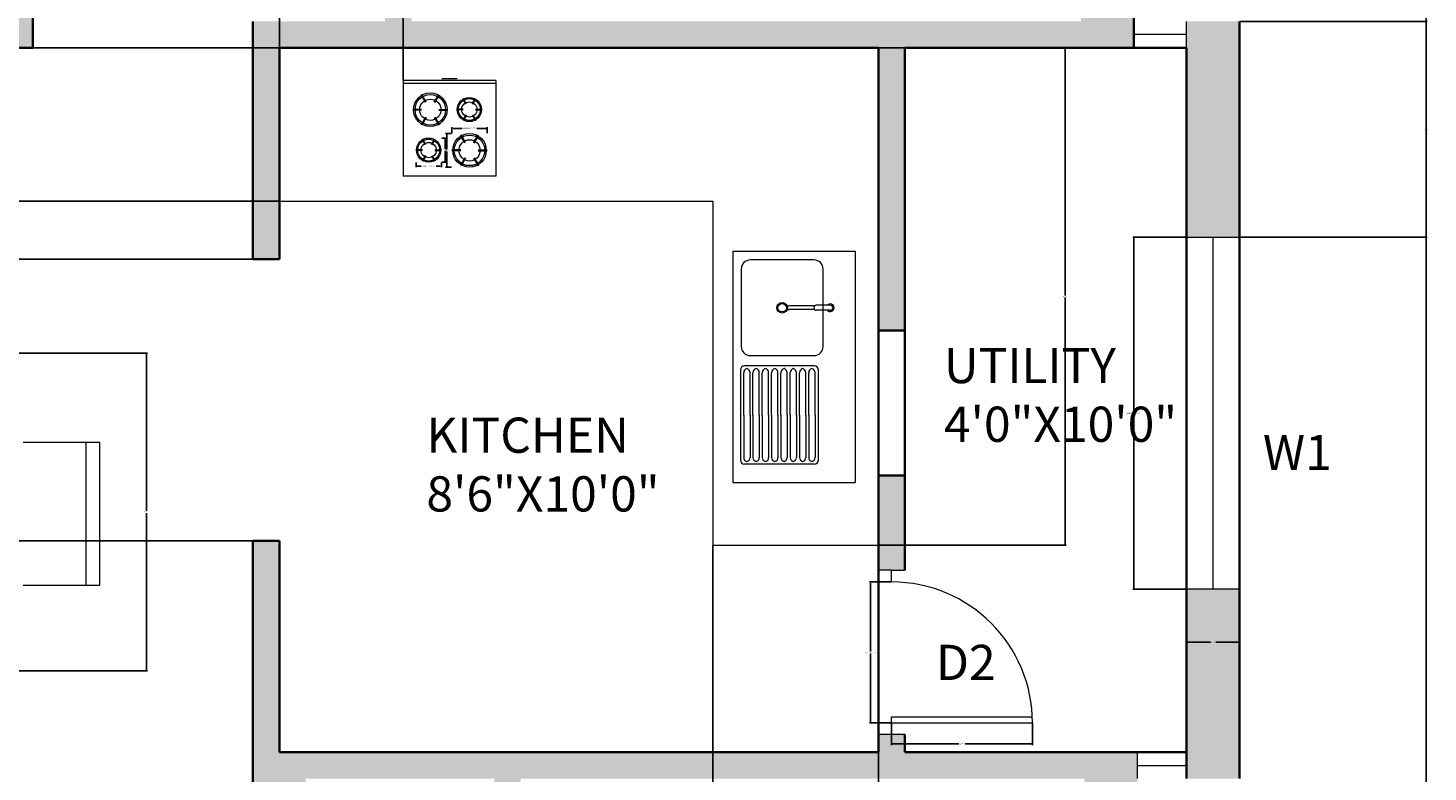
# Model space of a CAD drawing. Units: inches. Extents: x 5 to 421, y -617 to 43.
# Tile 13 of 15: x 182 to 421, y -246 to -119. Entities that reach past the tile are written whole.
import ezdxf

# ---------------------------------------------------------------- set-up
doc = ezdxf.new("R2010")
doc.units = ezdxf.units.IN
doc.header["$MEASUREMENT"] = 0
for name, color, linetype, lineweight in [('A-ANNO-DIMS', 2, 'Continuous', 18), ('A-ANNO-TEXT', 7, 'Continuous', 18), ('A-AREA-IDEN', 7, 'Continuous', 25), ('A-DOOR', 4, 'Continuous', 20), ('A-EQPM', 8, 'Continuous', 18), ('A-FLOR-CASE', 8, 'Continuous', 18), ('A-FLOR-FIXT', 9, 'Continuous', 18), ('A-FURN', 8, 'Continuous', 13), ('A-GLAZ', 4, 'Continuous', 18), ('A-WALL', 7, 'Continuous', 35)]:
    doc.layers.add(name, color=color, linetype=linetype, lineweight=lineweight)
doc.layers.add('A-WALL-PATT', color=251, linetype='Continuous', lineweight=13, true_color=0x636466)
doc.styles.get("Standard").update_dxf_attribs({"font": 'arial.ttf'})
doc.dimstyles.get("Standard").update_dxf_attribs({"dimtxt": 0.18, "dimasz": 0.18, "dimexe": 0.18, "dimexo": 0.0625, "dimgap": 0.09, "dimtad": 0, "dimtih": 1, "dimtoh": 1, "dimdec": 0, "dimzin": 0, "dimdsep": 46, "dimlunit": 3, "dimtxsty": 'Standard', "dimcen": 0.09, "dimadec": 0, "dimazin": 0, "dimtfac": 1, "dimtdec": 0, "dimtofl": 0, "dimtmove": 0, "dimatfit": 3, "dimfxl": 1, "dimtolj": 1, "dimtzin": 0, "dimarcsym": 0})

# ---------------------------------------------------------------- blocks, each defined once
blk = doc.blocks.new('WINDOW-W1-60')
for p, q in [((0, 9), (60, 9)), ((0, 0), (0, 9)), ((60, 9), (60, 0)), ((0, 4.5), (60, 4.5)), ((60, 0), (0, 0))]:
    blk.add_line(p, q)
blk = doc.blocks.new('DOOR-SWING-24')
for p, q in [((23, 0), (23, 24)), ((24, 0), (24, 24))]:
    blk.add_line(p, q)
blk.add_arc((24, 0), 24, 90, 180)
blk = doc.blocks.new('CHAIR-DINING')
for p, q in [((13.04, 24.35), (0, 24.35)), ((10.66, 24.35), (10.66, 0)), ((13.04, 0), (13.04, 24.35)), ((0, 0), (13.04, 0))]:
    blk.add_line(p, q)
blk = doc.blocks.new('BURNER-LARGE')
for p, q in [((2.2, 4.11), (1.44, 5.42)), ((2.31, 4.18), (1.55, 5.49)), ((3.68, 4.18), (4.44, 5.49)), ((3.79, 4.11), (4.55, 5.42)), ((1.51, 2.92), (0, 2.92)), ((1.51, 2.79), (0, 2.79)), ((4.48, 2.92), (5.99, 2.92)), ((4.48, 2.79), (5.99, 2.79)), ((2.2, 1.61), (1.44, 0.3)), ((2.31, 1.54), (1.55, 0.23)), ((3.68, 1.54), (4.44, 0.23)), ((3.79, 1.61), (4.55, 0.3))]:
    blk.add_line(p, q)
for radius in [2.86, 2.6, 1.81]:
    blk.add_circle((3, 2.86), radius)
blk = doc.blocks.new('BURNER-SMALL')
for p, q in [((1.58, 2.96), (1.04, 3.9)), ((1.66, 3.01), (1.12, 3.95)), ((2.65, 3.01), (3.19, 3.95)), ((2.73, 2.96), (3.28, 3.9)), ((1.09, 2.11), (0, 2.11)), ((1.09, 2.01), (0, 2.01)), ((1.58, 1.16), (1.04, 0.21)), ((1.66, 1.11), (1.12, 0.17)), ((2.65, 1.11), (3.19, 0.17)), ((2.73, 1.16), (3.28, 0.21)), ((3.22, 2.11), (4.31, 2.11)), ((3.22, 2.01), (4.31, 2.01))]:
    blk.add_line(p, q)
for radius in [2.06, 1.87, 1.3]:
    blk.add_circle((2.16, 2.06), radius)
blk = doc.blocks.new('*D18')
at = {"layer": 'A-ANNO-DIMS', "color": 0, "lineweight": -2, "transparency": 16777216}
for p, q in [((379.36, -154.87), (370.24, -154.87)), ((370.42, -155.05), (370.42, -184.69)), ((370.42, -214.69), (370.42, -185.05)), ((379.36, -214.87), (370.24, -214.87))]:
    blk.add_line(p, q, dxfattribs=at)
at = {"layer": 'A-ANNO-DIMS', "color": 0, "transparency": 16777216}
for points in [[(370.39, -155.05), (370.45, -155.05), (370.42, -154.87)], [(370.39, -214.69), (370.45, -214.69), (370.42, -214.87)]]:
    blk.add_solid(points, dxfattribs=at)
at = {"layer": 'Defpoints', "color": 0, "transparency": 16777216}
for p in [(370.42, -154.87), (379.42, -154.87), (379.42, -214.87)]:
    blk.add_point(p, dxfattribs=at)
at = {"layer": 'A-ANNO-DIMS', "color": 0, "transparency": 16777216, "insert": (370.42, -184.87), "char_height": 0.18, "attachment_point": 5}
blk.add_mtext('\\A1;WINDOW W1 60 TYP.', dxfattribs=at)
blk = doc.blocks.new('*D19')
at = {"layer": 'A-ANNO-DIMS', "color": 0, "lineweight": -2, "transparency": 16777216}
for p, q in [((379.42, -214.93), (379.42, -224.05)), ((388.42, -214.93), (388.42, -224.05)), ((379.6, -223.87), (383.46, -223.87)), ((388.24, -223.87), (384.38, -223.87))]:
    blk.add_line(p, q, dxfattribs=at)
at = {"layer": 'A-ANNO-DIMS', "color": 0, "transparency": 16777216}
for points in [[(379.6, -223.84), (379.6, -223.9), (379.42, -223.87)], [(388.24, -223.84), (388.24, -223.9), (388.42, -223.87)]]:
    blk.add_solid(points, dxfattribs=at)
at = {"layer": 'Defpoints', "color": 0, "transparency": 16777216}
for p in [(379.42, -214.87), (388.42, -214.87), (379.42, -223.87)]:
    blk.add_point(p, dxfattribs=at)
at = {"layer": 'A-ANNO-DIMS', "color": 0, "transparency": 16777216, "insert": (383.92, -223.87), "char_height": 0.18, "attachment_point": 5}
blk.add_mtext('\\A1;9 TYP.', dxfattribs=at)
blk = doc.blocks.new('*D22')
at = {"layer": 'A-ANNO-DIMS', "color": 0, "lineweight": -2, "transparency": 16777216}
for p, q in [((329.11, -213.62), (325.39, -213.62)), ((325.57, -213.8), (325.57, -225.44)), ((325.57, -237.44), (325.57, -225.8)), ((329.11, -237.62), (325.39, -237.62))]:
    blk.add_line(p, q, dxfattribs=at)
at = {"layer": 'A-ANNO-DIMS', "color": 0, "transparency": 16777216}
for points in [[(325.54, -213.8), (325.6, -213.8), (325.57, -213.62)], [(325.54, -237.44), (325.6, -237.44), (325.57, -237.62)]]:
    blk.add_solid(points, dxfattribs=at)
at = {"layer": 'Defpoints', "color": 0, "transparency": 16777216}
for p in [(329.17, -213.62), (325.57, -237.62), (329.17, -237.62)]:
    blk.add_point(p, dxfattribs=at)
at = {"layer": 'A-ANNO-DIMS', "color": 0, "transparency": 16777216, "insert": (325.57, -225.62), "char_height": 0.18, "attachment_point": 5}
blk.add_mtext('\\A1;DOOR D2 24 TYP.', dxfattribs=at)
blk = doc.blocks.new('*D23')
at = {"layer": 'A-ANNO-DIMS', "color": 0, "lineweight": -2, "transparency": 16777216}
for p, q in [((329.17, -237.68), (329.17, -241.4)), ((353.17, -237.68), (353.17, -241.4)), ((329.35, -241.22), (340.64, -241.22)), ((352.99, -241.22), (341.7, -241.22))]:
    blk.add_line(p, q, dxfattribs=at)
at = {"layer": 'A-ANNO-DIMS', "color": 0, "transparency": 16777216}
for points in [[(329.35, -241.19), (329.35, -241.25), (329.17, -241.22)], [(352.99, -241.19), (352.99, -241.25), (353.17, -241.22)]]:
    blk.add_solid(points, dxfattribs=at)
at = {"layer": 'Defpoints', "color": 0, "transparency": 16777216}
for p in [(329.17, -237.62), (353.17, -237.62), (353.17, -241.22)]:
    blk.add_point(p, dxfattribs=at)
at = {"layer": 'A-ANNO-DIMS', "color": 0, "transparency": 16777216, "insert": (341.17, -241.22), "char_height": 0.18, "attachment_point": 5}
blk.add_mtext('\\A1;24 TYP.', dxfattribs=at)
blk = doc.blocks.new('*D44')
at = {"layer": 'A-ANNO-DIMS', "color": 0, "lineweight": -2, "transparency": 16777216}
for p, q in [((254.31, -137.17), (254.31, -136.16)), ((254.49, -136.34), (256.04, -136.34)), ((260.12, -136.34), (258.57, -136.34)), ((260.3, -137.17), (260.3, -136.16))]:
    blk.add_line(p, q, dxfattribs=at)
at = {"layer": 'A-ANNO-DIMS', "color": 0, "transparency": 16777216}
for points in [[(254.49, -136.31), (254.49, -136.37), (254.31, -136.34)], [(260.12, -136.31), (260.12, -136.37), (260.3, -136.34)]]:
    blk.add_solid(points, dxfattribs=at)
at = {"layer": 'Defpoints', "color": 0, "transparency": 16777216}
for p in [(254.31, -136.34), (254.31, -137.23), (260.3, -137.23)]:
    blk.add_point(p, dxfattribs=at)
at = {"layer": 'A-ANNO-DIMS', "color": 0, "transparency": 16777216, "insert": (257.31, -136.34), "char_height": 0.18, "attachment_point": 5}
blk.add_mtext('\\A1;LARGE RING 6 TYP.', dxfattribs=at)
blk = doc.blocks.new('*D45')
at = {"layer": 'A-ANNO-DIMS', "color": 0, "lineweight": -2, "transparency": 16777216}
for p, q in [((254.25, -137.23), (253.23, -137.23)), ((253.41, -137.41), (253.41, -139.91)), ((253.41, -142.77), (253.41, -140.28)), ((254.25, -142.95), (253.23, -142.95))]:
    blk.add_line(p, q, dxfattribs=at)
at = {"layer": 'A-ANNO-DIMS', "color": 0, "transparency": 16777216}
for points in [[(253.38, -137.41), (253.44, -137.41), (253.41, -137.23)], [(253.38, -142.77), (253.44, -142.77), (253.41, -142.95)]]:
    blk.add_solid(points, dxfattribs=at)
at = {"layer": 'Defpoints', "color": 0, "transparency": 16777216}
for p in [(254.31, -137.23), (253.41, -142.95), (254.31, -142.95)]:
    blk.add_point(p, dxfattribs=at)
at = {"layer": 'A-ANNO-DIMS', "color": 0, "transparency": 16777216, "insert": (253.41, -140.09), "char_height": 0.18, "attachment_point": 5}
blk.add_mtext('\\A1;6 TYP.', dxfattribs=at)
blk = doc.blocks.new('*D46')
at = {"layer": 'A-ANNO-DIMS', "color": 0, "lineweight": -2, "transparency": 16777216}
for p, q in [((248.19, -142.17), (248.19, -142.94)), ((248.37, -142.76), (249.09, -142.76)), ((252.32, -142.76), (251.6, -142.76)), ((252.5, -142.17), (252.5, -142.94))]:
    blk.add_line(p, q, dxfattribs=at)
at = {"layer": 'A-ANNO-DIMS', "color": 0, "transparency": 16777216}
for points in [[(248.37, -142.73), (248.37, -142.79), (248.19, -142.76)], [(252.32, -142.73), (252.32, -142.79), (252.5, -142.76)]]:
    blk.add_solid(points, dxfattribs=at)
at = {"layer": 'Defpoints', "color": 0, "transparency": 16777216}
for p in [(248.19, -142.11), (248.19, -142.76), (252.5, -142.11)]:
    blk.add_point(p, dxfattribs=at)
at = {"layer": 'A-ANNO-DIMS', "color": 0, "transparency": 16777216, "insert": (250.34, -142.76), "char_height": 0.18, "attachment_point": 5}
blk.add_mtext('\\A1;SMALL RING 4 TYP.', dxfattribs=at)
blk = doc.blocks.new('*D47')
at = {"layer": 'A-ANNO-DIMS', "color": 0, "lineweight": -2, "transparency": 16777216}
for p, q in [((252.56, -137.99), (253.33, -137.99)), ((253.15, -138.17), (253.15, -139.87)), ((253.15, -141.93), (253.15, -140.23)), ((252.56, -142.11), (253.33, -142.11))]:
    blk.add_line(p, q, dxfattribs=at)
at = {"layer": 'A-ANNO-DIMS', "color": 0, "transparency": 16777216}
for points in [[(253.12, -138.17), (253.18, -138.17), (253.15, -137.99)], [(253.12, -141.93), (253.18, -141.93), (253.15, -142.11)]]:
    blk.add_solid(points, dxfattribs=at)
at = {"layer": 'Defpoints', "color": 0, "transparency": 16777216}
for p in [(252.5, -137.99), (252.5, -142.11), (253.15, -142.11)]:
    blk.add_point(p, dxfattribs=at)
at = {"layer": 'A-ANNO-DIMS', "color": 0, "transparency": 16777216, "insert": (253.15, -140.05), "char_height": 0.18, "attachment_point": 5}
blk.add_mtext('\\A1;4 TYP.', dxfattribs=at)
blk = doc.blocks.new('*D55')
at = {"layer": 'A-ANNO-DIMS', "color": 0, "lineweight": -2, "transparency": 16777216}
for p, q in [((370.48, 10.88), (420.4, 10.88)), ((420.22, 10.7), (420.22, -286.69)), ((420.22, -584.44), (420.22, -287.05)), ((169.48, -584.62), (420.4, -584.62))]:
    blk.add_line(p, q, dxfattribs=at)
at = {"layer": 'A-ANNO-DIMS', "color": 0, "transparency": 16777216}
for points in [[(420.19, 10.7), (420.25, 10.7), (420.22, 10.88)], [(420.19, -584.44), (420.25, -584.44), (420.22, -584.62)]]:
    blk.add_solid(points, dxfattribs=at)
at = {"layer": 'Defpoints', "color": 0, "transparency": 16777216}
for p in [(370.42, 10.88), (169.42, -584.62), (420.22, -584.62)]:
    blk.add_point(p, dxfattribs=at)
at = {"layer": 'A-ANNO-DIMS', "color": 0, "transparency": 16777216, "insert": (420.22, -286.87), "char_height": 0.18, "attachment_point": 5}
blk.add_mtext('\\A1;595.5', dxfattribs=at)
blk = doc.blocks.new('*D64')
at = {"layer": 'A-ANNO-DIMS', "color": 0, "lineweight": -2, "transparency": 16777216}
for p, q in [((388.48, -118.12), (420.4, -118.12)), ((420.22, -118.3), (420.22, -136.31)), ((420.22, -154.69), (420.22, -136.68)), ((388.48, -154.87), (420.4, -154.87))]:
    blk.add_line(p, q, dxfattribs=at)
at = {"layer": 'A-ANNO-DIMS', "color": 0, "transparency": 16777216}
for points in [[(420.19, -118.3), (420.25, -118.3), (420.22, -118.12)], [(420.19, -154.69), (420.25, -154.69), (420.22, -154.87)]]:
    blk.add_solid(points, dxfattribs=at)
at = {"layer": 'Defpoints', "color": 0, "transparency": 16777216}
for p in [(388.42, -118.12), (388.42, -154.87), (420.22, -154.87)]:
    blk.add_point(p, dxfattribs=at)
at = {"layer": 'A-ANNO-DIMS', "color": 0, "transparency": 16777216, "insert": (420.22, -136.49), "char_height": 0.18, "attachment_point": 5}
blk.add_mtext('\\A1;36.75', dxfattribs=at)
blk = doc.blocks.new('*D67')
at = {"layer": 'A-ANNO-DIMS', "color": 0, "lineweight": -2, "transparency": 16777216}
for p, q in [((220.36, -158.62), (5.44, -158.62)), ((5.62, -158.8), (5.62, -182.44)), ((5.62, -206.44), (5.62, -182.8)), ((220.36, -206.62), (5.44, -206.62))]:
    blk.add_line(p, q, dxfattribs=at)
at = {"layer": 'A-ANNO-DIMS', "color": 0, "transparency": 16777216}
for points in [[(5.59, -158.8), (5.65, -158.8), (5.62, -158.62)], [(5.59, -206.44), (5.65, -206.44), (5.62, -206.62)]]:
    blk.add_solid(points, dxfattribs=at)
at = {"layer": 'Defpoints', "color": 0, "transparency": 16777216}
for p in [(220.42, -158.62), (5.62, -206.62), (220.42, -206.62)]:
    blk.add_point(p, dxfattribs=at)
at = {"layer": 'A-ANNO-DIMS', "color": 0, "transparency": 16777216, "insert": (5.62, -182.62), "char_height": 0.18, "attachment_point": 5}
blk.add_mtext('\\A1;48', dxfattribs=at)
blk = doc.blocks.new('*D68')
at = {"layer": 'A-ANNO-DIMS', "color": 0, "lineweight": -2, "transparency": 16777216}
for p, q in [((224.86, -122.62), (5.44, -122.62)), ((5.62, -122.8), (5.62, -135.49)), ((5.62, -148.54), (5.62, -135.85)), ((224.86, -148.72), (5.44, -148.72))]:
    blk.add_line(p, q, dxfattribs=at)
at = {"layer": 'A-ANNO-DIMS', "color": 0, "transparency": 16777216}
for points in [[(5.59, -122.8), (5.65, -122.8), (5.62, -122.62)], [(5.59, -148.54), (5.65, -148.54), (5.62, -148.72)]]:
    blk.add_solid(points, dxfattribs=at)
at = {"layer": 'Defpoints', "color": 0, "transparency": 16777216}
for p in [(224.92, -122.62), (5.62, -148.72), (224.92, -148.72)]:
    blk.add_point(p, dxfattribs=at)
at = {"layer": 'A-ANNO-DIMS', "color": 0, "transparency": 16777216, "insert": (5.62, -135.67), "char_height": 0.18, "attachment_point": 5}
blk.add_mtext('\\A1;26.1', dxfattribs=at)
blk = doc.blocks.new('*D69')
at = {"layer": 'A-ANNO-DIMS', "color": 0, "lineweight": -2, "transparency": 16777216}
for p, q in [((298.73, -207.41), (298.73, -616.6)), ((326.92, -207.41), (326.92, -616.6)), ((298.91, -616.42), (312.43, -616.42)), ((326.74, -616.42), (313.22, -616.42))]:
    blk.add_line(p, q, dxfattribs=at)
at = {"layer": 'A-ANNO-DIMS', "color": 0, "transparency": 16777216}
for points in [[(298.91, -616.39), (298.91, -616.45), (298.73, -616.42)], [(326.74, -616.39), (326.74, -616.45), (326.92, -616.42)]]:
    blk.add_solid(points, dxfattribs=at)
at = {"layer": 'Defpoints', "color": 0, "transparency": 16777216}
for p in [(298.73, -207.35), (326.92, -207.35), (326.92, -616.42)]:
    blk.add_point(p, dxfattribs=at)
at = {"layer": 'A-ANNO-DIMS', "color": 0, "transparency": 16777216, "insert": (312.82, -616.42), "char_height": 0.18, "attachment_point": 5}
blk.add_mtext('\\A1;28.19', dxfattribs=at)
blk = doc.blocks.new('*D70')
at = {"layer": 'A-ANNO-DIMS', "color": 0, "lineweight": -2, "transparency": 16777216}
for p, q in [((326.98, -122.62), (358.9, -122.62)), ((358.72, -122.8), (358.72, -164.8)), ((358.72, -207.17), (358.72, -165.16)), ((326.98, -207.35), (358.9, -207.35))]:
    blk.add_line(p, q, dxfattribs=at)
at = {"layer": 'A-ANNO-DIMS', "color": 0, "transparency": 16777216}
for points in [[(358.69, -122.8), (358.75, -122.8), (358.72, -122.62)], [(358.69, -207.17), (358.75, -207.17), (358.72, -207.35)]]:
    blk.add_solid(points, dxfattribs=at)
at = {"layer": 'Defpoints', "color": 0, "transparency": 16777216}
for p in [(326.92, -122.62), (326.92, -207.35), (358.72, -207.35)]:
    blk.add_point(p, dxfattribs=at)
at = {"layer": 'A-ANNO-DIMS', "color": 0, "transparency": 16777216, "insert": (358.72, -164.98), "char_height": 0.18, "attachment_point": 5}
blk.add_mtext('\\A1;84.73', dxfattribs=at)
blk = doc.blocks.new('*D71')
at = {"layer": 'A-ANNO-DIMS', "color": 0, "lineweight": -2, "transparency": 16777216}
for p, q in [((224.92, -122.56), (224.92, 42.86)), ((225.1, 42.68), (235.06, 42.68)), ((245.82, 42.68), (235.85, 42.68)), ((246, -128.12), (246, 42.86))]:
    blk.add_line(p, q, dxfattribs=at)
at = {"layer": 'A-ANNO-DIMS', "color": 0, "transparency": 16777216}
for points in [[(225.1, 42.71), (225.1, 42.65), (224.92, 42.68)], [(245.82, 42.71), (245.82, 42.65), (246, 42.68)]]:
    blk.add_solid(points, dxfattribs=at)
at = {"layer": 'Defpoints', "color": 0, "transparency": 16777216}
for p in [(246, 42.68), (224.92, -122.62), (246, -128.18)]:
    blk.add_point(p, dxfattribs=at)
at = {"layer": 'A-ANNO-DIMS', "color": 0, "transparency": 16777216, "insert": (235.46, 42.68), "char_height": 0.18, "attachment_point": 5}
blk.add_mtext('\\A1;21.08', dxfattribs=at)
blk = doc.blocks.new('*D77')
at = {"layer": 'A-ANNO-DIMS', "color": 0, "lineweight": -2, "transparency": 16777216}
for p, q in [((170.53, -174.62), (202.45, -174.62)), ((202.27, -174.8), (202.27, -201.5)), ((202.27, -228.56), (202.27, -201.87)), ((170.53, -228.74), (202.45, -228.74))]:
    blk.add_line(p, q, dxfattribs=at)
at = {"layer": 'A-ANNO-DIMS', "color": 0, "transparency": 16777216}
for points in [[(202.24, -174.8), (202.3, -174.8), (202.27, -174.62)], [(202.24, -228.56), (202.3, -228.56), (202.27, -228.74)]]:
    blk.add_solid(points, dxfattribs=at)
at = {"layer": 'Defpoints', "color": 0, "transparency": 16777216}
for p in [(170.47, -174.62), (170.47, -228.74), (202.27, -228.74)]:
    blk.add_point(p, dxfattribs=at)
at = {"layer": 'A-ANNO-DIMS', "color": 0, "transparency": 16777216, "insert": (202.27, -201.68), "char_height": 0.18, "attachment_point": 5}
blk.add_mtext('\\A1;54.12', dxfattribs=at)

msp = doc.modelspace()

# ---------------------------------------------------------------- hatches: boundary and pattern name
at = {"layer": 'A-WALL-PATT'}
h = msp.add_hatch(color=256, dxfattribs=at)
h.dxf.hatch_style = 1
h.paths.add_polyline_path([(46.4196, -88.1188), (37.4196, -88.1188), (37.4196, -166.6119), (46.4196, -166.6119), (46.4196, -122.6188), (135.4196, -122.6188), (135.4196, -120.3688), (135.4196, -118.1188), (46.4196, -118.1188)])
h.paths.add_polyline_path([(82.4196, 10.8812), (37.4196, 10.8812), (37.4196, -28.1188), (46.4196, -28.1188), (46.4196, 1.8812), (82.4196, 1.8812)])
h.paths.add_polyline_path([(215.5968, 10.8812), (142.4196, 10.8812), (142.4196, 1.8812), (178.4196, 1.8812), (178.4196, -118.1188), (175.4196, -118.1188), (175.4196, -122.6188), (182.9196, -122.6188), (182.9196, -80.6188), (211.9196, -80.6188), (211.9196, -78.3688), (211.9196, -76.1188), (182.9196, -76.1188), (182.9196, 1.8812), (215.5968, 1.8812)])
h.paths.add_polyline_path([(274.4196, 10.8812), (239.5968, 10.8812), (239.5968, 1.8812), (242.9196, 1.8812), (242.9196, -76.1188), (239.9196, -76.1188), (239.9196, -80.6188), (242.9196, -80.6188), (242.9196, -83.6188), (247.4196, -83.6188), (247.4196, 1.8812), (274.4196, 1.8812)])
h.paths.add_polyline_path([(370.4196, 10.8812), (334.4196, 10.8812), (334.4196, 1.8812), (361.4196, 1.8812), (361.4196, -28.1188), (370.4196, -28.1188)])
h.paths.add_polyline_path([(370.4196, -88.1188), (361.4196, -88.1188), (361.4196, -118.1188), (247.4196, -118.1188), (247.4196, -115.1188), (242.9196, -115.1188), (242.9196, -118.1188), (220.4196, -118.1188), (220.4196, -158.6188), (224.9196, -158.6188), (224.9196, -122.6188), (326.9196, -122.6188), (326.9196, -170.7662), (331.4196, -170.7662), (331.4196, -122.6188), (370.4196, -122.6188)])
h.paths.add_polyline_path([(388.4196, -122.6188), (388.4196, -118.1188), (379.4196, -118.1188), (379.4196, -122.6188), (379.4196, -154.8688), (388.4196, -154.8688)])
h.paths.add_polyline_path([(388.4196, -214.8688), (379.4196, -214.8688), (379.4196, -247.1188), (388.4196, -247.1188)])
h.paths.add_polyline_path([(371.0265, -242.6188), (331.4196, -242.6188), (331.4196, -239.6188), (326.9196, -239.6188), (326.9196, -242.6188), (224.9196, -242.6188), (224.9196, -206.6188), (220.4196, -206.6188), (220.4196, -343.6188), (224.9196, -343.6188), (229.4196, -343.6188), (229.4196, -247.1188), (261.5265, -247.1188), (261.5265, -276.1188), (263.7765, -276.1188), (266.0265, -276.1188), (266.0265, -247.1188), (362.0265, -247.1188), (362.0265, -265.1188), (371.0265, -265.1188), (371.0265, -247.1188)])
h.paths.add_polyline_path([(371.0265, -289.1188), (362.0265, -289.1188), (362.0265, -307.1188), (266.0265, -307.1188), (266.0265, -304.1188), (261.5265, -304.1188), (261.5265, -307.1188), (261.5265, -311.6188), (362.0265, -311.6188), (362.0265, -353.6188), (371.0265, -353.6188)])
h.paths.add_polyline_path([(371.0265, -413.6188), (362.0265, -413.6188), (362.0265, -455.6188), (325.7231, -455.6188), (325.7231, -464.6188), (361.4196, -464.6188), (371.0265, -464.6188)])
h.paths.add_polyline_path([(265.7231, -455.6188), (229.4196, -455.6188), (229.4196, -383.6188), (220.4196, -383.6188), (220.4196, -386.6188), (207.4649, -386.6188), (207.4649, -395.6188), (220.4196, -395.6188), (220.4196, -455.6188), (216.0568, -455.6188), (216.0568, -464.6188), (265.7231, -464.6188)])
h.paths.add_polyline_path([(169.4196, -386.6188), (137.9196, -386.6188), (137.9196, -395.6188), (160.4196, -395.6188), (160.4196, -424.2032), (169.4196, -424.2032)])
h.paths.add_polyline_path([(169.4196, -453.7423), (160.4196, -453.7423), (160.4196, -464.6188), (169.4196, -464.6188)])
h.paths.add_polyline_path([(46.4196, -575.6188), (37.4196, -575.6188), (37.4196, -584.6188), (46.4196, -584.6188)])
h.paths.add_polyline_path([(169.4196, -575.6188), (160.4196, -575.6188), (160.4196, -579.5504), (160.4196, -584.6188), (169.4196, -584.6188)])
h.paths.add_polyline_path([(46.4196, -226.6119), (37.4196, -226.6119), (37.4196, -292.8008), (46.4196, -292.8008)])
h.paths.add_polyline_path([(46.4196, -352.8008), (37.4196, -352.8008), (37.4196, -395.6188), (77.9196, -395.6188), (77.9196, -386.6188), (46.4196, -386.6188)])
h = msp.add_hatch(color=256, dxfattribs=at)
h.dxf.hatch_style = 1
h.paths.add_polyline_path([(331.4196, -195.4945), (326.9196, -195.4945), (326.9196, -211.6188), (329.1696, -211.6188), (331.4196, -211.6188)])

# ---------------------------------------------------------------- linework, layer by layer
at = {"layer": 'A-DOOR'}
for p, q in [((329.1696, -211.6188), (326.9196, -211.6188)), ((329.1696, -213.6188), (329.1696, -211.6188)), ((329.1696, -211.6188), (331.4196, -211.6188)), ((329.1696, -239.6188), (329.1696, -236.6188)), ((331.4196, -239.6188), (326.9196, -239.6188))]:
    msp.add_line(p, q, dxfattribs=at)
at = {"layer": 'A-EQPM'}
for p, q in [((261.7704, -128.1837), (245.9983, -128.1837)), ((245.9983, -128.1837), (245.9983, -144.4815)), ((261.7704, -128.7094), (245.9983, -128.7094)), ((255.1987, -127.9208), (252.57, -127.9208)), ((261.7704, -128.1837), (261.7704, -144.4815)), ((261.7704, -144.4815), (245.9983, -144.4815))]:
    msp.add_line(p, q, dxfattribs=at)
at = {"layer": 'A-FLOR-CASE'}
for p, q in [((224.9196, -148.7194), (298.7283, -148.7194)), ((298.7283, -148.7194), (298.7283, -207.3464)), ((298.7283, -207.3464), (326.9196, -207.3464))]:
    msp.add_line(p, q, dxfattribs=at)
at = {"layer": 'A-FLOR-FIXT'}
for p, q in [((302.1261, -157.252), (322.9694, -157.252)), ((302.1261, -157.252), (302.1261, -196.6848)), ((322.9694, -157.252), (322.9694, -196.6848)), ((315.9609, -158.7608), (305.1288, -158.7608)), ((303.5763, -160.3132), (303.5763, -173.4968)), ((317.5134, -167.1449), (317.5134, -160.3132)), ((317.5134, -173.4968), (317.5134, -167.3362)), ((305.1288, -175.0492), (315.9609, -175.0492)), ((303.4193, -177.5307), (303.4193, -192.8379)), ((303.9907, -185.1843), (303.9907, -177.9626)), ((316.0034, -176.8119), (304.138, -176.8119)), ((305.0685, -185.1843), (305.0685, -177.9626)), ((305.5733, -185.1843), (305.5733, -177.9626)), ((306.6511, -185.1843), (306.6511, -177.9626)), ((307.1559, -185.1843), (307.1559, -177.9626)), ((308.2337, -185.1843), (308.2337, -177.9626)), ((308.7385, -185.1843), (308.7385, -177.9626)), ((309.8163, -185.1843), (309.8163, -177.9626)), ((310.3211, -185.1843), (310.3211, -177.9626)), ((311.3989, -185.1843), (311.3989, -177.9626)), ((311.9037, -185.1843), (311.9037, -177.9626)), ((312.9815, -185.1843), (312.9815, -177.9626)), ((313.4863, -185.1843), (313.4863, -177.9626)), ((314.564, -185.1843), (314.564, -177.9626)), ((315.0688, -185.1843), (315.0688, -177.9626)), ((316.1466, -185.1843), (316.1466, -177.9626)), ((316.7221, -192.8379), (316.7221, -177.5307)), ((303.9907, -185.1843), (303.9907, -192.406)), ((305.0685, -185.1843), (305.0685, -192.406)), ((305.5733, -185.1843), (305.5733, -192.406)), ((306.6511, -185.1843), (306.6511, -192.406)), ((307.1559, -185.1843), (307.1559, -192.406)), ((308.2337, -185.1843), (308.2337, -192.406)), ((308.7385, -185.1843), (308.7385, -192.406)), ((309.8163, -185.1843), (309.8163, -192.406)), ((310.3211, -185.1843), (310.3211, -192.406)), ((311.3989, -185.1843), (311.3989, -192.406)), ((311.9037, -185.1843), (311.9037, -192.406)), ((312.9815, -185.1843), (312.9815, -192.406)), ((313.4863, -185.1843), (313.4863, -192.406)), ((314.564, -185.1843), (314.564, -192.406)), ((315.0688, -185.1843), (315.0688, -192.406)), ((316.1466, -185.1843), (316.1466, -192.406)), ((316.0034, -193.5567), (304.138, -193.5567)), ((302.1261, -196.6848), (322.9694, -196.6848))]:
    msp.add_line(p, q, dxfattribs=at)
for points in [[(316.0868, -166.5816), (311.7229, -166.5816)], [(318.7246, -166.4738), (316.3558, -166.4738)], [(316.0868, -167.2284), (311.7229, -167.2284)], [(318.7246, -167.3362), (316.3558, -167.3362)]]:
    msp.add_lwpolyline(points, dxfattribs=at)
for radius in [0.8984, 0.7187]:
    msp.add_circle((310.5449, -166.905), radius, dxfattribs=at)
for centre, radius, start, end in [((305.1288, -160.3132), 1.5525, 90, 180), ((315.9609, -160.3132), 1.5525, 0, 90), ((311.6943, -166.905), 0.3247, 84.94633, 275.05367), ((316.3726, -166.905), 0.4316, 92.219765, 267.780235), ((318.7246, -166.905), 0.6457, 221.901781, 138.098219), ((318.7246, -166.905), 0.4312, 270, 90), ((305.1288, -173.4968), 1.5525, 180, 270), ((315.9609, -173.4968), 1.5525, 270, 0), ((304.138, -177.5307), 0.7187, 90, 180), ((304.7094, -177.9626), 0.7187, 104.490333, 180), ((304.3498, -177.9626), 0.7187, 0, 75.509667), ((306.292, -177.9626), 0.7187, 104.490333, 180), ((305.9323, -177.9626), 0.7187, 0, 75.509667), ((307.8746, -177.9626), 0.7187, 104.490333, 180), ((307.5149, -177.9626), 0.7187, 0, 75.509667), ((309.4572, -177.9626), 0.7187, 104.490333, 180), ((309.0975, -177.9626), 0.7187, 0, 75.509667), ((311.0398, -177.9626), 0.7187, 104.490333, 180), ((310.6801, -177.9626), 0.7187, 0, 75.509667), ((312.6224, -177.9626), 0.7187, 104.490333, 180), ((312.2627, -177.9626), 0.7187, 0, 75.509667), ((314.205, -177.9626), 0.7187, 104.490333, 180), ((313.8453, -177.9626), 0.7187, 0, 75.509667), ((315.7876, -177.9626), 0.7187, 104.490333, 180), ((315.4279, -177.9626), 0.7187, 0, 75.509667), ((316.0034, -177.5307), 0.7187, 0, 90), ((304.138, -192.8379), 0.7187, 180, 270), ((304.7094, -192.406), 0.7187, 180, 255.509667), ((304.3498, -192.406), 0.7187, 284.490333, 0), ((306.292, -192.406), 0.7187, 180, 255.509667), ((305.9323, -192.406), 0.7187, 284.490333, 0), ((307.8746, -192.406), 0.7187, 180, 255.509667), ((307.5149, -192.406), 0.7187, 284.490333, 0), ((309.4572, -192.406), 0.7187, 180, 255.509667), ((309.0975, -192.406), 0.7187, 284.490333, 0), ((311.0398, -192.406), 0.7187, 180, 255.509667), ((310.6801, -192.406), 0.7187, 284.490333, 0), ((312.6224, -192.406), 0.7187, 180, 255.509667), ((312.2627, -192.406), 0.7187, 284.490333, 0), ((314.205, -192.406), 0.7187, 180, 255.509667), ((313.8453, -192.406), 0.7187, 284.490333, 0), ((315.7876, -192.406), 0.7187, 180, 255.509667), ((315.4279, -192.406), 0.7187, 284.490333, 0), ((316.0034, -192.8379), 0.7187, 270, 0)]:
    msp.add_arc(centre, radius, start, end, dxfattribs=at)
at = {"layer": 'A-GLAZ'}
for p, q in [((379.4196, -122.6188), (379.4196, -118.1188)), ((379.4196, -120.3688), (370.4196, -120.3688)), ((371.0265, -247.1188), (371.0265, -242.6188)), ((371.0265, -244.8688), (379.4196, -244.8688))]:
    msp.add_line(p, q, dxfattribs=at)
at = {"layer": 'A-WALL'}
for p, q in [((370.4196, 10.8812), (370.4196, -122.6188)), ((182.9196, -80.6188), (182.9196, -122.6188)), ((220.4196, -118.1188), (220.4196, -158.6188)), ((388.4196, -118.1188), (388.4196, -122.6188)), ((46.4196, -122.6188), (182.9196, -122.6188)), ((224.9196, -122.6188), (326.9196, -122.6188)), ((224.9196, -122.6188), (224.9196, -158.6188)), ((326.9196, -122.6188), (326.9196, -242.6188)), ((331.4196, -122.6188), (331.4196, -211.6188)), ((331.4196, -122.6188), (379.4196, -122.6188)), ((379.4196, -122.6188), (379.4196, -247.1188)), ((388.4196, -122.6188), (388.4196, -247.1188)), ((224.9196, -158.6188), (220.4196, -158.6188)), ((326.9196, -170.7662), (331.4196, -170.7662)), ((326.9196, -195.4945), (331.4196, -195.4945)), ((224.9196, -206.6188), (220.4196, -206.6188)), ((220.4196, -206.6188), (220.4196, -386.6188)), ((224.9196, -206.6188), (224.9196, -242.6188)), ((331.4196, -239.6188), (331.4196, -242.6188)), ((224.9196, -242.6188), (326.9196, -242.6188)), ((331.4196, -242.6188), (379.4196, -242.6188))]:
    msp.add_line(p, q, dxfattribs=at)

# ---------------------------------------------------------------- block references
at = {"layer": 'A-DOOR', "rotation": 270}
msp.add_blockref('DOOR-SWING-24', (329.1696, -213.6188), dxfattribs=at)
at = {"layer": 'A-EQPM'}
for name, p in [('BURNER-LARGE', (247.6179, -136.0369)), ('BURNER-SMALL', (255.107, -135.1935))]:
    msp.add_blockref(name, p, dxfattribs=at)
at = {"layer": 'A-EQPM', "rotation": 180}
for name, p in [('BURNER-SMALL', (252.5, -137.9925)), ('BURNER-LARGE', (260.3011, -137.235))]:
    msp.add_blockref(name, p, dxfattribs=at)
at = {"layer": 'A-FURN'}
msp.add_blockref('CHAIR-DINING', (181.2958, -214.1862), dxfattribs=at)
at = {"layer": 'A-GLAZ', "rotation": 90.00000000000011}
msp.add_blockref('WINDOW-W1-60', (388.4196, -214.8688), dxfattribs=at)

# ---------------------------------------------------------------- texts
at = {"layer": 'A-ANNO-TEXT', "char_height": 6, "attachment_point": 1}
for s, insert in [('W1', (392.4042, -188.5696)), ('D2', (336.7234, -224.3201))]:
    msp.add_mtext(s, dxfattribs=dict(at, insert=insert))
at = {"layer": 'A-AREA-IDEN', "char_height": 6, "attachment_point": 1}
for s, insert in [('UTILITY\\P4\'0"X10\'0"', (338.0866, -173.7484)), ('KITCHEN\\P8\'6"X10\'0"', (249.9484, -185.6138))]:
    msp.add_mtext(s, dxfattribs=dict(at, insert=insert))

# ---------------------------------------------------------------- dimensions: what is measured, and where the dimension line sits
at = {"layer": 'A-ANNO-DIMS'}
for base, p1, p2, picture, middle in [((245.9983, 42.6812), (224.9196, -122.6188), (245.9983, -128.1837), '*D71', (235.4589, 42.6812)), ((326.9196, -616.4188), (298.7283, -207.3464), (326.9196, -207.3464), '*D69', (312.8239, -616.4188))]:
    dim = msp.add_linear_dim(base=base, p1=p1, p2=p2, dimstyle='Standard', override={"dimdec": 2, "dimlfac": 1, "dimrnd": 0, "dimzin": 0, "dimdsep": 46, "dimlunit": 2}, dxfattribs=at)
    dim.commit()
    dim.dimension.update_dxf_attribs({"geometry": picture, "text_midpoint": middle})
for base, p1, p2, angle, override, picture, middle in [((420.2196, -584.6188), (370.4196, 10.8812), (169.4196, -584.6188), 90, {"dimdec": 1, "dimlfac": 1, "dimrnd": 0, "dimzin": 0, "dimdsep": 46, "dimlunit": 2}, '*D55', (420.2196, -286.8688)), ((420.2196, -154.8688), (388.4196, -118.1188), (388.4196, -154.8688), 90, {"dimdec": 2, "dimlfac": 1, "dimrnd": 0, "dimzin": 0, "dimdsep": 46, "dimlunit": 2}, '*D64', (420.2196, -136.4938)), ((5.6196, -148.7194), (224.9196, -122.6188), (224.9196, -148.7194), 90, {"dimdec": 1, "dimlfac": 1, "dimrnd": 0, "dimzin": 0, "dimdsep": 46, "dimlunit": 2}, '*D68', (5.6196, -135.6691)), ((358.7196, -207.3464), (326.9196, -122.6188), (326.9196, -207.3464), 270, {"dimdec": 2, "dimlfac": 1, "dimrnd": 0, "dimzin": 0, "dimdsep": 46, "dimlunit": 2}, '*D70', (358.7196, -164.9826)), ((5.6196, -206.6188), (220.4196, -158.6188), (220.4196, -206.6188), 90, {"dimdec": 0, "dimlfac": 1, "dimrnd": 0, "dimzin": 0, "dimdsep": 46, "dimlunit": 2}, '*D67', (5.6196, -182.6188)), ((202.2715, -228.745), (170.4715, -174.6231), (170.4715, -228.745), 270, {"dimdec": 2, "dimlfac": 1, "dimrnd": 0, "dimzin": 0, "dimdsep": 46, "dimlunit": 2}, '*D77', (202.2715, -201.684))]:
    dim = msp.add_linear_dim(base=base, p1=p1, p2=p2, angle=angle, dimstyle='Standard', override=override, dxfattribs=at)
    dim.commit()
    dim.dimension.update_dxf_attribs({"geometry": picture, "text_midpoint": middle})
for base, p1, p2, angle, text, picture, middle in [((254.3105, -136.3364), (260.3011, -137.235), (254.3105, -137.235), 180, 'LARGE RING <> TYP.', '*D44', (257.3058, -136.3364)), ((253.147, -142.1091), (252.5, -137.9925), (252.5, -142.1091), 270, '<> TYP.', '*D47', (253.147, -140.0508)), ((253.4119, -142.9524), (254.3105, -137.235), (254.3105, -142.9524), 270, '<> TYP.', '*D45', (253.4119, -140.0937)), ((248.1868, -142.756), (252.5, -142.1091), (248.1868, -142.1091), 180, 'SMALL RING <> TYP.', '*D46', (250.3434, -142.756)), ((370.4196, -154.8688), (379.4196, -214.8688), (379.4196, -154.8688), 90, 'WINDOW W1 <> TYP.', '*D18', (370.4196, -184.8688)), ((325.5696, -237.6188), (329.1696, -213.6188), (329.1696, -237.6188), 270, 'DOOR D2 <> TYP.', '*D22', (325.5696, -225.6188)), ((379.4196, -223.8688), (388.4196, -214.8688), (379.4196, -214.8688), 180, '<> TYP.', '*D19', (383.9196, -223.8688))]:
    dim = msp.add_linear_dim(base=base, p1=p1, p2=p2, angle=angle, text=text, dimstyle='Standard', override={"dimdec": 0, "dimlfac": 1, "dimrnd": 0, "dimzin": 0, "dimdsep": 46, "dimlunit": 2}, dxfattribs=at)
    dim.commit()
    dim.dimension.update_dxf_attribs({"geometry": picture, "text_midpoint": middle})
dim = msp.add_linear_dim(base=(353.1696, -241.2188), p1=(329.1696, -237.6188), p2=(353.1696, -237.6188), text='<> TYP.', dimstyle='Standard', override={"dimdec": 0, "dimlfac": 1, "dimrnd": 0, "dimzin": 0, "dimdsep": 46, "dimlunit": 2}, dxfattribs=at)
dim.commit()
dim.dimension.update_dxf_attribs({"geometry": '*D23', "text_midpoint": (341.1696, -241.2188)})

doc.saveas('drawing.dxf')
